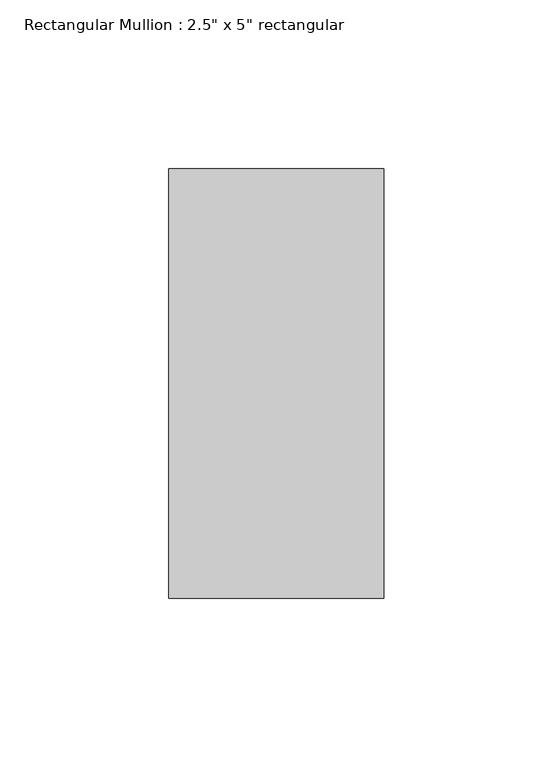
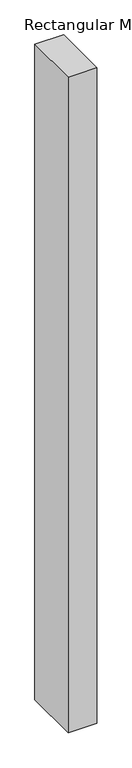
"""IFC4 building model written with IfcOpenShell, lengths in millimetres: member geometry."""

from ifc_helpers import new_model, si_unit, frame, origin, place, context, project, spatial, polyline, outline, extrude, source, transform, mapped, element, save


def member_49b269a4(model_context):
    return source(origin(), model_context, "Body", "SweptSolid", [
        extrude(outline(polyline([(31.75, 63.5), (31.75, -63.5), (-31.75, -63.5), (-31.75, 63.5), (31.75, 63.5)])), frame((0.0, 0.0, -1532.0284144), z_axis=(0.0, 0.0, 1.0), x_axis=(1.0, 0.0, 0.0)), (0.0, 0.0, 1.0), 1532.0284144),
    ])


if __name__ == "__main__":
    model = new_model("IFC4")
    model_context = context("Model", 3, world=origin())
    ifc_project = project(units=[si_unit("LENGTHUNIT", "METRE", prefix="MILLI")], contexts=[model_context])
    site = spatial("IfcSite", under=ifc_project)
    building = spatial("IfcBuilding", under=site)
    placement = place(None, origin())
    member_shape = member_49b269a4(model_context)
    element("IfcMember", 1, ObjectType="Rectangular Mullion : 2.5\" x 5\" rectangular", at=placement, inside=building, context=model_context, shape_type="MappedRepresentation", body=[
        mapped(member_shape, transform((0.0, 0.0, 0.0), x_axis=(1.0, 0.0, 0.0), y_axis=(0.0, 1.0, 0.0), z_axis=(0.0, 0.0, 1.0))),
    ])
    save(model, "model.ifc")

# Revit data of these elements
# Type "Rectangular Mullion : 2.5\" x 5\" rectangular"
#   built-in parameter 1007304 = 0.416667 (stored number, unit not read)
#   built-in parameter 1007301 = 0.104167 (stored number, unit not read)
#   built-in parameter 1007300 = 0.104167 (stored number, unit not read)
# Element 1 (IfcMember, "Rectangular Mullion : 2.5\" x 5\" rectangular")
#   Materials on its faces: "Aluminum"
# Materials
#   "Aluminum": class "Metal", colour RGB 247 247 247, transparency 0, Description = "Aluminum 6061", Cost = 0
